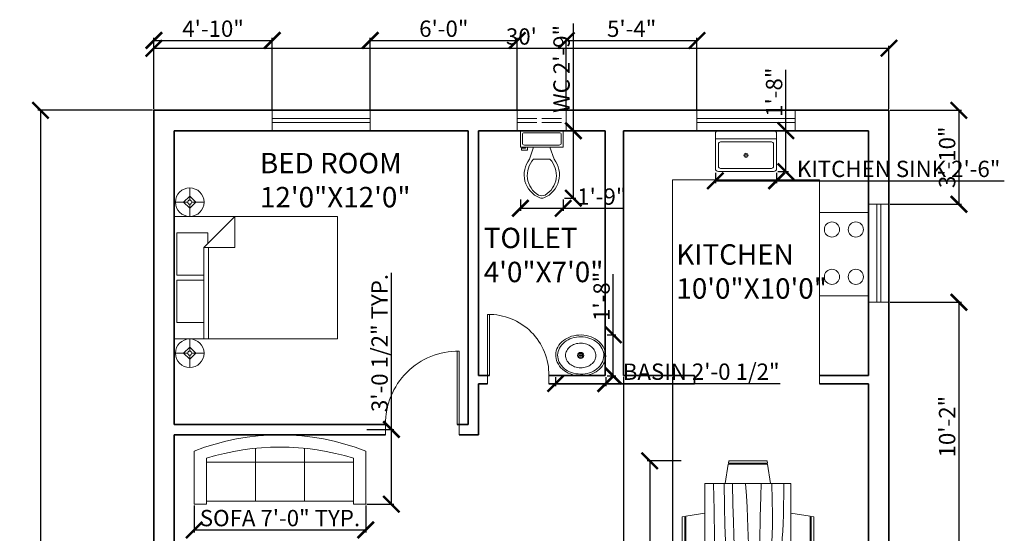
# Model space of a CAD drawing. Units: inches. Extents: x 21865 to 22885, y 36660 to 37408.
# Tile 4 of 6: x 21865 to 22347, y 37157 to 37408. Entities that reach past the tile are written whole.
import ezdxf

# ---------------------------------------------------------------- set-up
doc = ezdxf.new("R2010")
doc.units = ezdxf.units.IN
doc.linetypes.add('ACAD_ISO02W100', pattern=[15, 12, -3])
for name, color, linetype, lineweight in [('A-ANNO-DIMS', 2, 'Continuous', 18), ('A-AREA-IDEN', 7, 'Continuous', 20), ('A-DOOR', 3, 'Continuous', 20), ('A-EQPM', 9, 'Continuous', 18), ('A-FLOR-CASE', 8, 'Continuous', 20), ('A-FLOR-FIXT', 9, 'Continuous', 18), ('A-FURN', 8, 'Continuous', 18), ('A-GLAZ', 4, 'Continuous', 18), ('A-GLAZ-OVHD', 4, 'ACAD_ISO02W100', 18), ('A-WALL', 7, 'Continuous', 35)]:
    doc.layers.add(name, color=color, linetype=linetype, lineweight=lineweight)
doc.styles.get("Standard").update_dxf_attribs({"font": 'arial.ttf'})
doc.dimstyles.new('ISO-25', dxfattribs={"dimtxt": 8, "dimasz": 8, "dimexe": 1.25, "dimexo": 0.625, "dimtad": 1, "dimlunit": 3, "dimtxsty": 'Standard', "dimblk": 'ARCHTICK', "dimcen": 2.5, "dimclrd": 4, "dimclre": 5, "dimclrt": 1, "dimadec": 0, "dimazin": 0, "dimtfac": 1, "dimtmove": 0, "dimatfit": 3, "dimfxl": 1, "dimarcsym": 0})

# ---------------------------------------------------------------- blocks, each defined once
blk = doc.blocks.new('Sink - Oval top')
for p, q in [((-1, 0), (1, 0)), ((0, 1), (0, -1))]:
    blk.add_line(p, q)
for points in [[(-12.23, 0.39, 0.117634), (-11.46, -3.36, 0.104469), (-8.88, -6.8, 0.090016), (-5.08, -9.07, 0.08192), (-0.32, -10.02, 0.08192), (4.49, -9.38, 0.090016), (8.42, -7.36, 0.104469), (11.22, -4.09, 0.117634), (12.23, -0.39, 0.117634), (11.46, 3.36, 0.104469), (8.88, 6.8, 0.090016), (5.08, 9.07, 0.08192), (0.32, 10.02, 0.08192), (-4.49, 9.38, 0.090016), (-8.42, 7.36, 0.104469), (-11.22, 4.09, 0.117634)], [(-11.29, 0.16, 0.118622), (-10.52, -3.25, 0.104678), (-8.07, -6.36, 0.089562), (-4.54, -8.37, 0.081185), (-0.13, -9.15, 0.081185), (4.3, -8.49, 0.089562), (7.89, -6.58, 0.104678), (10.42, -3.55, 0.118622), (11.29, -0.16, 0.118622), (10.52, 3.25, 0.104678), (8.07, 6.36, 0.089562), (4.54, 8.37, 0.081185), (0.13, 9.15, 0.081185), (-4.3, 8.49, 0.089562), (-7.89, 6.58, 0.104678), (-10.42, 3.55, 0.118622)], [(-7.42, 0.08, 0.118283), (-6.91, -2.17, 0.104607), (-5.29, -4.21, 0.089718), (-2.97, -5.53, 0.081436), (-0.07, -6.04, 0.081436), (2.84, -5.59, 0.089718), (5.2, -4.33, 0.104607), (6.86, -2.32, 0.118283), (7.42, -0.08, 0.118283), (6.91, 2.17, 0.104607), (5.29, 4.21, 0.089718), (2.97, 5.53, 0.081436), (0.07, 6.04, 0.081436), (-2.84, 5.59, 0.089718), (-5.2, 4.33, 0.104607), (-6.86, 2.32, 0.118283)]]:
    blk.add_lwpolyline(points, format="xyb", close=True)
for radius in [1.5, 1]:
    blk.add_circle((0, 0), radius)
blk = doc.blocks.new('Toilet - top')
for p, q in [((9.5, -6), (9.5, -2)), ((-10, -8.5), (-8, -8.5)), ((-10, -9.5), (-10, -8.5)), ((-7, -9.5), (-10, -9.5)), ((-8, -8.5), (-8, -8)), ((-7, -8), (-7, -9.5)), ((-4, -8), (-6, -14)), ((4, -8), (6, -14)), ((4, -14), (-4, -14))]:
    blk.add_line(p, q)
blk.add_lwpolyline([(10.5, -8), (10.5, 0), (-10.5, 0), (-10.5, -8)], close=True)
for points in [[(-9.5, -2), (-9.5, -6)], [(8.5, -1), (-8.5, -1)], [(-8.5, -7), (8.5, -7)]]:
    blk.add_lwpolyline(points)
for centre, radius, start, end in [((-8.62, -1.88), 0.884, 81.8699, 188.1301), ((8.62, -1.88), 0.884, 351.8699, 98.1301), ((-8.62, -6.12), 0.884, 171.8699, 278.1301), ((8.62, -6.12), 0.884, 261.8699, 8.1301), ((3.52, -21.58), 12.17, 141.4691, 247.9714), ((4.2, -21.82), 11.33, 136.3677, 238.9468), ((-3.52, -21.58), 12.17, 292.0284, 38.5307), ((-4.2, -21.82), 11.33, 301.053, 43.6321), ((0, -27.88), 4, 245.7318, 294.2682), ((0, -29), 4, 254.8605, 285.1395)]:
    blk.add_arc(centre, radius, start, end)
blk = doc.blocks.new('Sink-single - 30 in top')
blk.add_line((-15, -3.999996), (15, -3.999996))
for points in [[(-13.5, 0), (13.5, 0)], [(-15, -18.499996), (-15, -1.5)], [(15, -1.5), (15, -18.499996)], [(-13.5, -17.499996), (-13.5, -6.499996)], [(-12.5, -5.499996), (12.5, -5.499996)], [(13.5, -6.499996), (13.5, -17.499996)], [(12.5, -18.499996), (-12.5, -18.499996)], [(13.5, -19.999996), (-13.5, -19.999996)]]:
    blk.add_lwpolyline(points)
for radius in [1, 0.5]:
    blk.add_circle((0, -11.999996), radius)
for centre, radius, start, end in [((-13.5, -1.5), 1.5, 90, 180), ((13.5, -1.5), 1.5, 0, 90), ((-12.5, -6.499996), 1, 90, 180), ((12.5, -6.499996), 1, 0, 90), ((-13.5, -18.499996), 1.5, 180, 270), ((-12.5, -17.499996), 1, 180, 270), ((12.5, -17.499996), 1, 270, 0), ((13.5, -18.499996), 1.5, 270, 0)]:
    blk.add_arc(centre, radius, start, end)
blk = doc.blocks.new('Sofa - Roundback 7 ft.')
for p, q in [((-12.00002, -32.4421), (-12.00003, -6.5971)), ((11.99997, -32.4421), (11.99998, -6.5971)), ((-36.000027, -34), (-36.000027, -11.4696)), ((-35.999844, -13.3819), (35.9998, -13.3819)), ((35.99998, -34), (35.99998, -11.4696)), ((-36.000027, -32.4421), (35.99998, -32.4421))]:
    blk.add_line(p, q)
for points in [[(-36.000027, -34), (-42.000027, -34), (-42.000027, -8)], [(41.99998, -8), (41.99998, -34), (35.99998, -34)]]:
    blk.add_lwpolyline(points)
for centre, radius, start, end in [((0, -114.25), 114.25, 68.43141, 111.5686), ((-0.00001, -127.1968), 121.1968, 72.72033, 107.2797)]:
    blk.add_arc(centre, radius, start, end)
blk = doc.blocks.new('Dining Set - 36 x 72 in.')
for p, q in [((-22.2343, 26.00059), (-23.4847, 17.99762)), ((-22.2304, 26), (-5.7608, 26)), ((-22, 27.5), (-22.1562, 26.50042)), ((-5.8416, 26.5), (-22.1534, 26.5)), ((-22, 27.5), (-6, 27.5)), ((-5.8437, 26.49966), (-6, 27.5)), ((-4.5152, 17.99762), (-5.7655, 25.99926)), ((5.7657, 26.00059), (4.5153, 17.99762)), ((5.7696, 26), (22.2392, 26)), ((6, 27.5), (5.8438, 26.50042)), ((22.1584, 26.5), (5.8466, 26.5)), ((6, 27.5), (22, 27.5)), ((22.1563, 26.49966), (22, 27.5)), ((23.4848, 17.99762), (22.2345, 25.99926)), ((36, 18), (-36, 18)), ((-36, 18), (-36, -18)), ((36, -18), (36, 18)), ((-44.0006, 8.23428), (-35.9976, 9.48474)), ((44.0006, 8.23428), (35.9976, 9.48474)), ((-45.5, 8), (-44.5004, 8.15617)), ((-45.5, 8), (-45.5, -8)), ((-44.5, -8.15843), (-44.5, 8.15338)), ((-44, 8.23041), (-44, -8.23915)), ((44, 8.23041), (44, -8.23915)), ((44.5, -8.15843), (44.5, 8.15338)), ((45.5, 8), (44.5005, 8.15617)), ((45.5, 8), (45.5, -8)), ((-44.4997, -8.15631), (-45.5, -8)), ((-35.9976, -9.48476), (-43.9993, -8.2345)), ((35.9976, -9.48476), (43.9993, -8.2345)), ((44.4997, -8.15631), (45.5, -8)), ((-36, -18), (36, -18)), ((-22.2343, -26.0006), (-23.4847, -17.99762)), ((-4.5152, -17.99762), (-5.7655, -25.99928)), ((5.7657, -26.0006), (4.5153, -17.99762)), ((23.4848, -17.99762), (22.2345, -25.99928)), ((-22.2304, -26), (-5.7608, -26)), ((-22, -27.5), (-22.1562, -26.50044)), ((-5.8416, -26.5), (-22.1534, -26.5)), ((-22, -27.5), (-6, -27.5)), ((-5.8437, -26.49967), (-6, -27.5)), ((5.7696, -26), (22.2392, -26)), ((6, -27.5), (5.8438, -26.50044)), ((22.1584, -26.5), (5.8466, -26.5)), ((6, -27.5), (22, -27.5)), ((22.1563, -26.49967), (22, -27.5))]:
    blk.add_line(p, q)
for points in [[(-36, 15), (-31.1772, 14.97754), (-26.8079, 14.91406), (-22.8538, 14.81543), (-19.276, 14.6875), (-16.0362, 14.53613), (-13.0957, 14.36718), (-10.4159, 14.18652), (-7.9583, 14), (-5.6904, 13.81315), (-3.6035, 13.63021), (-1.6954, 13.45508), (0.0365, 13.29166), (1.5945, 13.14388), (2.9811, 13.01562), (4.1988, 12.9108), (5.25, 12.83333), (6.1393, 12.78613), (6.8802, 12.76823), (7.4883, 12.77767), (7.9792, 12.8125), (8.3685, 12.87077), (8.6719, 12.95052), (8.9049, 13.0498), (9.0833, 13.16666), (9.2205, 13.29899), (9.3216, 13.44401), (9.3895, 13.59879), (9.4271, 13.76041), (9.4373, 13.92594), (9.4232, 14.09245), (9.3875, 14.257), (9.3333, 14.41666), (9.2638, 14.56917), (9.1836, 14.71484), (9.0975, 14.85465), (9.0104, 14.98958), (8.9272, 15.1206), (8.8529, 15.2487), (8.7922, 15.37483), (8.75, 15.5), (8.7305, 15.62467), (8.7344, 15.74739), (8.7617, 15.86621), (8.8125, 15.97916), (8.8867, 16.08431), (8.9844, 16.17968), (9.1055, 16.26334), (9.25, 16.33333), (9.4189, 16.38802), (9.6172, 16.42708), (9.8506, 16.45052), (10.125, 16.45833), (10.4463, 16.45052), (10.8203, 16.42708), (11.2529, 16.38802), (11.75, 16.33333), (12.3184, 16.26318), (12.9694, 16.17838), (13.7151, 16.07991), (14.5677, 15.96875), (15.5395, 15.84586), (16.6426, 15.71224), (17.8893, 15.56884), (19.2917, 15.41666), (20.859, 15.25667), (22.5879, 15.08984), (24.4721, 14.91715), (26.5052, 14.73958), (28.6809, 14.5581), (30.9929, 14.3737), (33.4347, 14.18733), (36, 14)], [(-36, 10), (-28.9766, 10.14274), (-23.1725, 10.20442), (-18.4241, 10.19775), (-14.5677, 10.13541), (-11.4399, 10.03011), (-8.877, 9.89453), (-6.7154, 9.74137), (-4.7917, 9.58333), (-2.9698, 9.43082), (-1.2246, 9.28515), (0.4415, 9.14534), (2.026, 9.01041), (3.5266, 8.87939), (4.9408, 8.7513), (6.266, 8.62516), (7.5, 8.5), (8.6411, 8.37549), (9.6914, 8.2539), (10.6538, 8.13818), (11.5312, 8.03125), (12.3267, 7.93603), (13.043, 7.85547), (13.6831, 7.79248), (14.25, 7.75), (14.7471, 7.7303), (15.1797, 7.73307), (15.5537, 7.75732), (15.875, 7.80208), (16.1494, 7.86637), (16.3828, 7.94922), (16.5811, 8.04964), (16.75, 8.16666), (16.8944, 8.29915), (17.0143, 8.44531), (17.1089, 8.60319), (17.1771, 8.77083), (17.218, 8.94629), (17.2305, 9.1276), (17.2137, 9.31282), (17.1667, 9.5), (17.0895, 9.6875), (16.987, 9.875), (16.8649, 10.0625), (16.7292, 10.25), (16.5856, 10.4375), (16.4401, 10.625), (16.2985, 10.8125), (16.1667, 11), (16.05, 11.18733), (15.9518, 11.3737), (15.8752, 11.5581), (15.8229, 11.73958), (15.798, 11.91715), (15.8034, 12.08984), (15.842, 12.25667), (15.9167, 12.41666), (16.0295, 12.56836), (16.1784, 12.70833), (16.3605, 12.83268), (16.5729, 12.9375), (16.8127, 13.01888), (17.0768, 13.07291), (17.3625, 13.0957), (17.6667, 13.08333), (17.9894, 13.03312), (18.3418, 12.94726), (18.7382, 12.82918), (19.1927, 12.68229), (19.7195, 12.51001), (20.3327, 12.31575), (21.0465, 12.10294), (21.875, 11.875), (22.8357, 11.63354), (23.959, 11.37304), (25.2786, 11.08618), (26.8282, 10.76562), (28.6414, 10.40405), (30.752, 9.99414), (33.1936, 9.52856), (36, 9)], [(-36, 5.5), (-30.7157, 5.3348), (-26.069, 5.20963), (-21.9946, 5.11767), (-18.4271, 5.05208), (-15.3009, 5.00602), (-12.5508, 4.97265), (-10.1112, 4.94515), (-7.9167, 4.91666), (-5.909, 4.88167), (-4.0586, 4.83984), (-2.3429, 4.79215), (-0.7396, 4.73958), (0.7739, 4.6831), (2.22, 4.6237), (3.6213, 4.56233), (5, 4.5), (6.373, 4.43782), (7.7344, 4.3776), (9.0723, 4.32129), (10.375, 4.27083), (11.6309, 4.22819), (12.8281, 4.19531), (13.9551, 4.17415), (15, 4.16666), (15.954, 4.17448), (16.819, 4.19791), (17.6001, 4.23698), (18.3021, 4.29166), (18.9299, 4.36198), (19.4883, 4.44791), (19.9823, 4.54948), (20.4167, 4.66666), (20.7969, 4.79899), (21.1302, 4.94401), (21.4245, 5.09879), (21.6875, 5.26041), (21.9271, 5.42594), (22.1511, 5.59245), (22.3672, 5.757), (22.5834, 5.91666), (22.8065, 6.06868), (23.0404, 6.21093), (23.2879, 6.34147), (23.5521, 6.45833), (23.8358, 6.55957), (24.142, 6.64323), (24.4735, 6.70735), (24.8334, 6.75), (25.2235, 6.76969), (25.642, 6.76692), (26.0858, 6.74267), (26.5521, 6.69791), (27.0379, 6.63362), (27.5404, 6.55078), (28.0565, 6.45036), (28.5834, 6.33333), (29.1242, 6.19987), (29.7071, 6.04687), (30.3661, 5.87044), (31.1354, 5.66666), (32.0493, 5.43164), (33.142, 5.16146), (34.4475, 4.85221), (36, 4.5)], [(-36, -1), (-30.7915, -0.6591), (-26.0195, -0.38216), (-21.6519, -0.16284), (-17.6563, 0.00521), (-14.0005, 0.12833), (-10.6523, 0.21289), (-7.5796, 0.26522), (-4.75, 0.29166), (-2.134, 0.29793), (0.2878, 0.28711), (2.5317, 0.26163), (4.6146, 0.22396), (6.5529, 0.17651), (8.3633, 0.12174), (10.0623, 0.06209), (11.6667, 0), (13.1899, -0.06201), (14.6341, -0.1211), (15.9982, -0.17432), (17.2813, -0.21875), (18.4823, -0.25147), (19.6003, -0.26953), (20.6343, -0.27002), (21.5834, -0.25), (22.4481, -0.20768), (23.2357, -0.14584), (23.9549, -0.06836), (24.6146, 0.02083), (25.2235, 0.11784), (25.7904, 0.21875), (26.3241, 0.31966), (26.8334, 0.41666), (27.3265, 0.50618), (27.8099, 0.58593), (28.2894, 0.65397), (28.7709, 0.70833), (29.2601, 0.74707), (29.763, 0.76823), (30.2855, 0.76985), (30.8334, 0.75), (31.4088, 0.70784), (31.9994, 0.64713), (32.589, 0.57275), (33.1615, 0.48958), (33.7008, 0.4025), (34.1908, 0.3164), (34.6153, 0.23616), (34.9584, 0.16666), (35.2099, 0.11165), (35.3848, 0.07031), (35.504, 0.04069), (35.5886, 0.02083), (35.6594, 0.00879), (35.7377, 0.0026), (35.8442, 0.00032), (36, 0)], [(-36, -6.5), (-27.1843, -6.31267), (-20.084, -6.1263), (-14.469, -5.9419), (-10.1094, -5.76042), (-6.7752, -5.58285), (-4.2363, -5.41016), (-2.2629, -5.24333), (-0.625, -5.08334), (0.8708, -4.93099), (2.2715, -4.78646), (3.5872, -4.64974), (4.8281, -4.52084), (6.0046, -4.39974), (7.127, -4.28646), (8.2053, -4.18099), (9.25, -4.08334), (10.2705, -3.99382), (11.2734, -3.91407), (12.2647, -3.84603), (13.25, -3.79167), (14.2354, -3.75293), (15.2266, -3.73177), (16.2295, -3.73015), (17.25, -3.75), (18.2912, -3.79248), (19.3451, -3.85547), (20.4009, -3.93604), (21.4479, -4.03125), (22.4754, -4.13819), (23.4727, -4.25391), (24.4289, -4.37549), (25.3334, -4.5), (26.1785, -4.62492), (26.9694, -4.74935), (27.7145, -4.87281), (28.4219, -4.99479), (29.1, -5.11483), (29.7572, -5.23242), (30.4016, -5.34709), (31.0417, -5.45834), (31.6837, -5.56437), (32.3262, -5.65821), (32.9658, -5.73153), (33.599, -5.77604), (34.2224, -5.78345), (34.8327, -5.74545), (35.4264, -5.65373), (36, -5.5)], [(-36, -10), (-26.4022, -9.81299), (-18.4675, -9.62891), (-11.9839, -9.45069), (-6.7396, -9.28125), (-2.5226, -9.12354), (0.8789, -8.98047), (3.6769, -8.85498), (6.0833, -8.75), (8.2767, -8.66765), (10.3021, -8.60677), (12.1712, -8.56543), (13.8958, -8.54167), (15.4876, -8.53353), (16.9583, -8.53907), (18.3197, -8.55632), (19.5834, -8.58334), (20.7616, -8.61841), (21.8685, -8.66081), (22.9188, -8.71004), (23.9271, -8.76563), (24.9081, -8.82707), (25.8763, -8.89388), (26.8465, -8.96558), (27.8334, -9.04167), (28.8474, -9.12118), (29.8828, -9.20117), (30.93, -9.27824), (31.9792, -9.34896), (33.0205, -9.40991), (34.0443, -9.45768), (35.0407, -9.48885), (36, -9.5)], [(-36, -14.5), (-30.0881, -14.33513), (-25.0332, -14.21224), (-20.7312, -14.12647), (-17.0781, -14.07292), (-13.97, -14.04671), (-11.3027, -14.04297), (-8.9724, -14.05681), (-6.875, -14.08334), (-4.9224, -14.11833), (-3.0905, -14.16016), (-1.3709, -14.20785), (0.2448, -14.26042), (1.7647, -14.3169), (3.1973, -14.3763), (4.5507, -14.43767), (5.8333, -14.5), (7.0554, -14.5621), (8.235, -14.62175), (9.3922, -14.67652), (10.5469, -14.72396), (11.7192, -14.76164), (12.929, -14.78711), (14.1965, -14.79794), (15.5417, -14.79167), (16.9933, -14.76424), (18.6152, -14.70508), (20.4804, -14.60197), (22.6615, -14.44271), (25.2312, -14.21509), (28.2624, -13.9069), (31.8277, -13.50594), (36, -13)]]:
    blk.add_lwpolyline(points)
blk = doc.blocks.new('Bed - Queen')
for p, q in [((0, -80.00003), (0, 0)), ((0, 0), (59.99999, 0)), ((59.99999, 0), (59.99999, -80.00003)), ((7.99999, -1.2), (28.79998, -1.2)), ((7.99999, -14.4), (7.99999, -1.2)), ((28.79998, -1.2), (28.79998, -14.4)), ((31.19999, -1.2), (51.99999, -1.2)), ((31.19999, -14.4), (31.19999, -1.2)), ((51.99999, -1.2), (51.99999, -16.4)), ((0, -14.4), (44.8, -14.4)), ((59.99999, -29.6), (44.8, -14.4)), ((44.8, -14.4), (44.8, -29.6)), ((44.8, -16.8), (0, -16.8)), ((51.99999, -16.4), (46.79936, -16.4)), ((44.8, -29.6), (59.99999, -29.6)), ((59.99999, -80.00003), (0, -80.00003))]:
    blk.add_line(p, q)
blk = doc.blocks.new('Lamp - Table')
for p, q in [((0, 7), (0, 1)), ((-1, 0), (-7, 0)), ((0, 3), (-3, 0)), ((-3, 0), (0, -3)), ((3, 0), (0, 3)), ((0, -3), (3, 0)), ((1, 0), (7, 0)), ((0, -1), (0, -7))]:
    blk.add_line(p, q)
for radius in [7, 1]:
    blk.add_circle((0, 0), radius)
blk = doc.blocks.new('new block')
for name, p in [('Lamp - Table', (-35.8, -6.38)), ('Bed - Queen', (-28.8, 1.2))]:
    blk.add_blockref(name, p)
at = {"xscale": -1}
blk.add_blockref('Lamp - Table', (38.2, -6.38), dxfattribs=at)
blk = doc.blocks.new('_ArchTick')
at = {"color": 0, "linetype": 'ByBlock', "const_width": 0.15}
blk.add_lwpolyline([(-0.5, -0.5), (0.5, 0.5)], dxfattribs=at)
blk = doc.blocks.new('*D21')
at = {"layer": 'A-ANNO-DIMS', "color": 0, "lineweight": -2, "transparency": 16777216}
for p, q in [((21930.43, 37364.56), (21930.43, 37395.61)), ((21930.43, 37394.36), (22290.43, 37394.36)), ((22290.43, 37364.56), (22290.43, 37395.61))]:
    blk.add_line(p, q, dxfattribs=at)
at = {"layer": 'Defpoints', "color": 0, "transparency": 16777216}
for p in [(22290.43, 37394.36), (21930.43, 37363.93), (22290.43, 37363.93)]:
    blk.add_point(p, dxfattribs=at)
at = {"layer": 'A-ANNO-DIMS', "color": 0, "lineweight": -2, "transparency": 16777216, "xscale": 8, "yscale": 8, "zscale": 8, "rotation": 180}
blk.add_blockref('_ArchTick', (21930.43, 37394.36), dxfattribs=at)
at = {"layer": 'A-ANNO-DIMS', "color": 0, "lineweight": -2, "transparency": 16777216, "xscale": 8, "yscale": 8, "zscale": 8}
blk.add_blockref('_ArchTick', (22290.43, 37394.36), dxfattribs=at)
at = {"layer": 'A-ANNO-DIMS', "color": 0, "transparency": 16777216, "insert": (22110.43, 37399.07), "char_height": 8, "attachment_point": 5}
blk.add_mtext("30'", dxfattribs=at)
blk = doc.blocks.new('*D22')
at = {"layer": 'A-ANNO-DIMS', "color": 0, "lineweight": -2, "transparency": 16777216}
for p, q in [((21929.8, 37363.93), (21873.63, 37363.93)), ((21874.88, 37363.93), (21874.88, 36883.93)), ((21929.8, 36883.93), (21873.63, 36883.93))]:
    blk.add_line(p, q, dxfattribs=at)
at = {"layer": 'Defpoints', "color": 0, "transparency": 16777216}
for p in [(21930.43, 37363.93), (21874.88, 36883.93), (21930.43, 36883.93)]:
    blk.add_point(p, dxfattribs=at)
at = {"layer": 'A-ANNO-DIMS', "color": 0, "lineweight": -2, "transparency": 16777216, "xscale": 8, "yscale": 8, "zscale": 8}
for p, rotation in [((21874.88, 37363.93), 90), ((21874.88, 36883.93), 270)]:
    blk.add_blockref('_ArchTick', p, dxfattribs=dict(at, rotation=rotation))
at = {"layer": 'A-ANNO-DIMS', "color": 0, "transparency": 16777216, "insert": (21870.17, 37123.93), "char_height": 8, "attachment_point": 5, "rotation": 90}
blk.add_mtext("40'", dxfattribs=at)
blk = doc.blocks.new('WIN-W-48-PLAN')
for p, q in [((0, 0), (0, 10)), ((48, 0), (48, 10)), ((48, 6), (0, 6)), ((48, 4), (0, 4))]:
    blk.add_line(p, q)
blk = doc.blocks.new('DOOR-D1-36-PLAN')
for p, q in [((0, 36), (0, 41)), ((36, 36), (36, 41)), ((35, 36), (35, 0)), ((36, 36), (36, 0))]:
    blk.add_line(p, q)
blk.add_arc((35.5, 35.5), 35.5, 179.1931, 270.8069)
blk = doc.blocks.new('*D32')
at = {"layer": 'A-ANNO-DIMS', "color": 5, "lineweight": -2, "transparency": 16777216}
for p, q in [((21950.18, 37170.31), (21950.18, 37157.08)), ((22034.18, 37170.31), (22034.18, 37157.08))]:
    blk.add_line(p, q, dxfattribs=at)
at = {"layer": 'A-ANNO-DIMS', "color": 4, "lineweight": -2, "transparency": 16777216}
blk.add_line((21950.18, 37158.33), (22034.18, 37158.33), dxfattribs=at)
at = {"layer": 'Defpoints', "color": 0, "transparency": 16777216}
for p in [(21950.18, 37170.93), (22034.18, 37170.93), (22034.18, 37158.33)]:
    blk.add_point(p, dxfattribs=at)
at = {"layer": 'A-ANNO-DIMS', "color": 4, "lineweight": -2, "transparency": 16777216, "xscale": 8, "yscale": 8, "zscale": 8, "rotation": 180}
blk.add_blockref('_ArchTick', (21950.18, 37158.33), dxfattribs=at)
at = {"layer": 'A-ANNO-DIMS', "color": 4, "lineweight": -2, "transparency": 16777216, "xscale": 8, "yscale": 8, "zscale": 8}
blk.add_blockref('_ArchTick', (22034.18, 37158.33), dxfattribs=at)
at = {"layer": 'A-ANNO-DIMS', "color": 1, "transparency": 16777216, "insert": (21992.18, 37163.1), "char_height": 8, "attachment_point": 5}
blk.add_mtext('SOFA 7\'-0" TYP.', dxfattribs=at)
blk = doc.blocks.new('*D33')
at = {"layer": 'A-ANNO-DIMS', "color": 4, "lineweight": -2, "transparency": 16777216}
for p, q in [((22046.78, 37207.6), (22046.78, 37284.25)), ((22046.78, 37170.93), (22046.78, 37207.6))]:
    blk.add_line(p, q, dxfattribs=at)
at = {"layer": 'A-ANNO-DIMS', "color": 5, "lineweight": -2, "transparency": 16777216}
for p, q in [((22034.8, 37207.6), (22048.03, 37207.6)), ((22034.8, 37170.93), (22048.03, 37170.93))]:
    blk.add_line(p, q, dxfattribs=at)
at = {"layer": 'Defpoints', "color": 0, "transparency": 16777216}
for p in [(22034.18, 37207.6), (22046.78, 37207.6), (22034.18, 37170.93)]:
    blk.add_point(p, dxfattribs=at)
at = {"layer": 'A-ANNO-DIMS', "color": 4, "lineweight": -2, "transparency": 16777216, "xscale": 8, "yscale": 8, "zscale": 8}
for p, rotation in [((22046.78, 37207.6), 90), ((22046.78, 37170.93), 270)]:
    blk.add_blockref('_ArchTick', p, dxfattribs=dict(at, rotation=rotation))
at = {"layer": 'A-ANNO-DIMS', "color": 1, "transparency": 16777216, "insert": (22042.02, 37249.92), "char_height": 8, "attachment_point": 5, "rotation": 90}
blk.add_mtext('3\'-0 1/2" TYP.', dxfattribs=at)
blk = doc.blocks.new('*D42')
at = {"layer": 'A-ANNO-DIMS', "color": 5, "lineweight": -2, "transparency": 16777216}
for p, q in [((22127.21, 37233.13), (22127.21, 37228.83)), ((22151.76, 37233.13), (22151.76, 37228.83))]:
    blk.add_line(p, q, dxfattribs=at)
at = {"layer": 'A-ANNO-DIMS', "color": 4, "lineweight": -2, "transparency": 16777216}
for p, q in [((22127.21, 37230.08), (22151.76, 37230.08)), ((22151.76, 37230.08), (22237.21, 37230.08))]:
    blk.add_line(p, q, dxfattribs=at)
at = {"layer": 'Defpoints', "color": 0, "transparency": 16777216}
for p in [(22127.21, 37233.76), (22151.76, 37233.76), (22151.76, 37230.08)]:
    blk.add_point(p, dxfattribs=at)
at = {"layer": 'A-ANNO-DIMS', "color": 4, "lineweight": -2, "transparency": 16777216, "xscale": 8, "yscale": 8, "zscale": 8, "rotation": 180}
blk.add_blockref('_ArchTick', (22127.21, 37230.08), dxfattribs=at)
at = {"layer": 'A-ANNO-DIMS', "color": 4, "lineweight": -2, "transparency": 16777216, "xscale": 8, "yscale": 8, "zscale": 8}
blk.add_blockref('_ArchTick', (22151.76, 37230.08), dxfattribs=at)
at = {"layer": 'A-ANNO-DIMS', "color": 1, "transparency": 16777216, "insert": (22198.48, 37234.84), "char_height": 8, "attachment_point": 5}
blk.add_mtext('BASIN 2\'-0 1/2"', dxfattribs=at)
blk = doc.blocks.new('*D43')
at = {"layer": 'A-ANNO-DIMS', "color": 4, "lineweight": -2, "transparency": 16777216}
for p, q in [((22155.44, 37253.9), (22155.44, 37283.66)), ((22155.44, 37233.76), (22155.44, 37253.9))]:
    blk.add_line(p, q, dxfattribs=at)
at = {"layer": 'A-ANNO-DIMS', "color": 5, "lineweight": -2, "transparency": 16777216}
for p, q in [((22152.38, 37253.9), (22156.69, 37253.9)), ((22152.38, 37233.76), (22156.69, 37233.76))]:
    blk.add_line(p, q, dxfattribs=at)
at = {"layer": 'Defpoints', "color": 0, "transparency": 16777216}
for p in [(22151.76, 37253.9), (22155.44, 37253.9), (22151.76, 37233.76)]:
    blk.add_point(p, dxfattribs=at)
at = {"layer": 'A-ANNO-DIMS', "color": 4, "lineweight": -2, "transparency": 16777216, "xscale": 8, "yscale": 8, "zscale": 8}
for p, rotation in [((22155.44, 37253.9), 90), ((22155.44, 37233.76), 270)]:
    blk.add_blockref('_ArchTick', p, dxfattribs=dict(at, rotation=rotation))
at = {"layer": 'A-ANNO-DIMS', "color": 1, "transparency": 16777216, "insert": (22150.73, 37272.78), "char_height": 8, "attachment_point": 5, "rotation": 90}
blk.add_mtext('1\'-8"', dxfattribs=at)
blk = doc.blocks.new('*D44')
at = {"layer": 'A-ANNO-DIMS', "color": 4, "lineweight": -2, "transparency": 16777216}
for p, q in [((22135.89, 37353.93), (22135.89, 37406.5)), ((22135.89, 37320.89), (22135.89, 37353.93))]:
    blk.add_line(p, q, dxfattribs=at)
at = {"layer": 'A-ANNO-DIMS', "color": 5, "lineweight": -2, "transparency": 16777216}
for p, q in [((22131.55, 37353.93), (22137.14, 37353.93)), ((22131.55, 37320.89), (22137.14, 37320.89))]:
    blk.add_line(p, q, dxfattribs=at)
at = {"layer": 'Defpoints', "color": 0, "transparency": 16777216}
for p in [(22130.93, 37353.93), (22135.89, 37353.93), (22130.93, 37320.89)]:
    blk.add_point(p, dxfattribs=at)
at = {"layer": 'A-ANNO-DIMS', "color": 4, "lineweight": -2, "transparency": 16777216, "xscale": 8, "yscale": 8, "zscale": 8}
for p, rotation in [((22135.89, 37353.93), 90), ((22135.89, 37320.89), 270)]:
    blk.add_blockref('_ArchTick', p, dxfattribs=dict(at, rotation=rotation))
at = {"layer": 'A-ANNO-DIMS', "color": 1, "transparency": 16777216, "insert": (22131.13, 37384.22), "char_height": 8, "attachment_point": 5, "rotation": 90}
blk.add_mtext('WC 2\'-9"', dxfattribs=at)
blk = doc.blocks.new('*D45')
at = {"layer": 'A-ANNO-DIMS', "color": 5, "lineweight": -2, "transparency": 16777216}
for p, q in [((22109.93, 37320.26), (22109.93, 37314.68)), ((22130.93, 37320.26), (22130.93, 37314.68))]:
    blk.add_line(p, q, dxfattribs=at)
at = {"layer": 'A-ANNO-DIMS', "color": 4, "lineweight": -2, "transparency": 16777216}
for p, q in [((22109.93, 37315.93), (22130.93, 37315.93)), ((22130.93, 37315.93), (22160.69, 37315.93))]:
    blk.add_line(p, q, dxfattribs=at)
at = {"layer": 'Defpoints', "color": 0, "transparency": 16777216}
for p in [(22109.93, 37320.89), (22130.93, 37320.89), (22130.93, 37315.93)]:
    blk.add_point(p, dxfattribs=at)
at = {"layer": 'A-ANNO-DIMS', "color": 4, "lineweight": -2, "transparency": 16777216, "xscale": 8, "yscale": 8, "zscale": 8, "rotation": 180}
blk.add_blockref('_ArchTick', (22109.93, 37315.93), dxfattribs=at)
at = {"layer": 'A-ANNO-DIMS', "color": 4, "lineweight": -2, "transparency": 16777216, "xscale": 8, "yscale": 8, "zscale": 8}
blk.add_blockref('_ArchTick', (22130.93, 37315.93), dxfattribs=at)
at = {"layer": 'A-ANNO-DIMS', "color": 1, "transparency": 16777216, "insert": (22149.81, 37320.64), "char_height": 8, "attachment_point": 5}
blk.add_mtext('1\'-9"', dxfattribs=at)
blk = doc.blocks.new('*D46')
at = {"layer": 'A-ANNO-DIMS', "color": 5, "lineweight": -2, "transparency": 16777216}
for p, q in [((22205.43, 37333.31), (22205.43, 37328.18)), ((22235.43, 37333.31), (22235.43, 37328.18))]:
    blk.add_line(p, q, dxfattribs=at)
at = {"layer": 'A-ANNO-DIMS', "color": 4, "lineweight": -2, "transparency": 16777216}
for p, q in [((22205.43, 37329.43), (22235.43, 37329.43)), ((22235.43, 37329.43), (22346.94, 37329.43))]:
    blk.add_line(p, q, dxfattribs=at)
at = {"layer": 'Defpoints', "color": 0, "transparency": 16777216}
for p in [(22205.43, 37333.93), (22235.43, 37333.93), (22235.43, 37329.43)]:
    blk.add_point(p, dxfattribs=at)
at = {"layer": 'A-ANNO-DIMS', "color": 4, "lineweight": -2, "transparency": 16777216, "xscale": 8, "yscale": 8, "zscale": 8, "rotation": 180}
blk.add_blockref('_ArchTick', (22205.43, 37329.43), dxfattribs=at)
at = {"layer": 'A-ANNO-DIMS', "color": 4, "lineweight": -2, "transparency": 16777216, "xscale": 8, "yscale": 8, "zscale": 8}
blk.add_blockref('_ArchTick', (22235.43, 37329.43), dxfattribs=at)
at = {"layer": 'A-ANNO-DIMS', "color": 1, "transparency": 16777216, "insert": (22295.18, 37334.19), "char_height": 8, "attachment_point": 5}
blk.add_mtext('KITCHEN SINK 2\'-6"', dxfattribs=at)
blk = doc.blocks.new('*D47')
at = {"layer": 'A-ANNO-DIMS', "color": 4, "lineweight": -2, "transparency": 16777216}
for p, q in [((22239.93, 37353.93), (22239.93, 37383.69)), ((22239.93, 37333.93), (22239.93, 37353.93))]:
    blk.add_line(p, q, dxfattribs=at)
at = {"layer": 'A-ANNO-DIMS', "color": 5, "lineweight": -2, "transparency": 16777216}
for p, q in [((22236.05, 37353.93), (22241.18, 37353.93)), ((22236.05, 37333.93), (22241.18, 37333.93))]:
    blk.add_line(p, q, dxfattribs=at)
at = {"layer": 'Defpoints', "color": 0, "transparency": 16777216}
for p in [(22235.43, 37353.93), (22239.93, 37353.93), (22235.43, 37333.93)]:
    blk.add_point(p, dxfattribs=at)
at = {"layer": 'A-ANNO-DIMS', "color": 4, "lineweight": -2, "transparency": 16777216, "xscale": 8, "yscale": 8, "zscale": 8}
for p, rotation in [((22239.93, 37353.93), 90), ((22239.93, 37333.93), 270)]:
    blk.add_blockref('_ArchTick', p, dxfattribs=dict(at, rotation=rotation))
at = {"layer": 'A-ANNO-DIMS', "color": 1, "transparency": 16777216, "insert": (22235.22, 37372.81), "char_height": 8, "attachment_point": 5, "rotation": 90}
blk.add_mtext('1\'-8"', dxfattribs=at)
blk = doc.blocks.new('*D48')
at = {"layer": 'A-ANNO-DIMS', "color": 5, "lineweight": -2, "transparency": 16777216}
for p, q in [((22188.6, 37192.23), (22172.01, 37192.23)), ((22188.6, 37085.76), (22172.01, 37085.76))]:
    blk.add_line(p, q, dxfattribs=at)
at = {"layer": 'A-ANNO-DIMS', "color": 4, "lineweight": -2, "transparency": 16777216}
for p, q in [((22173.26, 37192.23), (22173.26, 37085.76)), ((22173.26, 37085.76), (22173.26, 36963.72))]:
    blk.add_line(p, q, dxfattribs=at)
at = {"layer": 'Defpoints', "color": 0, "transparency": 16777216}
for p in [(22189.23, 37192.23), (22173.26, 37085.76), (22189.23, 37085.76)]:
    blk.add_point(p, dxfattribs=at)
at = {"layer": 'A-ANNO-DIMS', "color": 4, "lineweight": -2, "transparency": 16777216, "xscale": 8, "yscale": 8, "zscale": 8}
for p, rotation in [((22173.26, 37192.23), 90), ((22173.26, 37085.76), 270)]:
    blk.add_blockref('_ArchTick', p, dxfattribs=dict(at, rotation=rotation))
at = {"layer": 'A-ANNO-DIMS', "color": 1, "transparency": 16777216, "insert": (22168.49, 37020.74), "char_height": 8, "attachment_point": 5, "rotation": 90}
blk.add_mtext('DINING SET 8\'-10 1/2"', dxfattribs=at)
blk = doc.blocks.new('*D52')
at = {"layer": 'A-ANNO-DIMS', "color": 5, "lineweight": -2, "transparency": 16777216}
for p, q in [((21930.43, 37364.56), (21930.43, 37399.43)), ((21988.43, 37364.56), (21988.43, 37399.43))]:
    blk.add_line(p, q, dxfattribs=at)
at = {"layer": 'A-ANNO-DIMS', "color": 4, "lineweight": -2, "transparency": 16777216}
blk.add_line((21930.43, 37398.18), (21988.43, 37398.18), dxfattribs=at)
at = {"layer": 'Defpoints', "color": 0, "transparency": 16777216}
for p in [(21988.43, 37398.18), (21930.43, 37363.93), (21988.43, 37363.93)]:
    blk.add_point(p, dxfattribs=at)
at = {"layer": 'A-ANNO-DIMS', "color": 4, "lineweight": -2, "transparency": 16777216, "xscale": 8, "yscale": 8, "zscale": 8, "rotation": 180}
blk.add_blockref('_ArchTick', (21930.43, 37398.18), dxfattribs=at)
at = {"layer": 'A-ANNO-DIMS', "color": 4, "lineweight": -2, "transparency": 16777216, "xscale": 8, "yscale": 8, "zscale": 8}
blk.add_blockref('_ArchTick', (21988.43, 37398.18), dxfattribs=at)
at = {"layer": 'A-ANNO-DIMS', "color": 1, "transparency": 16777216, "insert": (21959.43, 37402.89), "char_height": 8, "attachment_point": 5}
blk.add_mtext('4\'-10"', dxfattribs=at)
blk = doc.blocks.new('*D53')
at = {"layer": 'A-ANNO-DIMS', "color": 5, "lineweight": -2, "transparency": 16777216}
for p, q in [((22036.43, 37364.56), (22036.43, 37399.43)), ((22108.43, 37364.56), (22108.43, 37399.43))]:
    blk.add_line(p, q, dxfattribs=at)
at = {"layer": 'A-ANNO-DIMS', "color": 4, "lineweight": -2, "transparency": 16777216}
blk.add_line((22036.43, 37398.18), (22108.43, 37398.18), dxfattribs=at)
at = {"layer": 'Defpoints', "color": 0, "transparency": 16777216}
for p in [(22108.43, 37398.18), (22036.43, 37363.93), (22108.43, 37363.93)]:
    blk.add_point(p, dxfattribs=at)
at = {"layer": 'A-ANNO-DIMS', "color": 4, "lineweight": -2, "transparency": 16777216, "xscale": 8, "yscale": 8, "zscale": 8, "rotation": 180}
blk.add_blockref('_ArchTick', (22036.43, 37398.18), dxfattribs=at)
at = {"layer": 'A-ANNO-DIMS', "color": 4, "lineweight": -2, "transparency": 16777216, "xscale": 8, "yscale": 8, "zscale": 8}
blk.add_blockref('_ArchTick', (22108.43, 37398.18), dxfattribs=at)
at = {"layer": 'A-ANNO-DIMS', "color": 1, "transparency": 16777216, "insert": (22072.43, 37402.89), "char_height": 8, "attachment_point": 5}
blk.add_mtext('6\'-0"', dxfattribs=at)
blk = doc.blocks.new('*D54')
at = {"layer": 'A-ANNO-DIMS', "color": 5, "lineweight": -2, "transparency": 16777216}
for p, q in [((22132.43, 37364.56), (22132.43, 37399.43)), ((22196.43, 37364.56), (22196.43, 37399.43))]:
    blk.add_line(p, q, dxfattribs=at)
at = {"layer": 'A-ANNO-DIMS', "color": 4, "lineweight": -2, "transparency": 16777216}
blk.add_line((22132.43, 37398.18), (22196.43, 37398.18), dxfattribs=at)
at = {"layer": 'Defpoints', "color": 0, "transparency": 16777216}
for p in [(22196.43, 37398.18), (22132.43, 37363.93), (22196.43, 37363.93)]:
    blk.add_point(p, dxfattribs=at)
at = {"layer": 'A-ANNO-DIMS', "color": 4, "lineweight": -2, "transparency": 16777216, "xscale": 8, "yscale": 8, "zscale": 8, "rotation": 180}
blk.add_blockref('_ArchTick', (22132.43, 37398.18), dxfattribs=at)
at = {"layer": 'A-ANNO-DIMS', "color": 4, "lineweight": -2, "transparency": 16777216, "xscale": 8, "yscale": 8, "zscale": 8}
blk.add_blockref('_ArchTick', (22196.43, 37398.18), dxfattribs=at)
at = {"layer": 'A-ANNO-DIMS', "color": 1, "transparency": 16777216, "insert": (22164.43, 37402.87), "char_height": 8, "attachment_point": 5}
blk.add_mtext('5\'-4"', dxfattribs=at)
blk = doc.blocks.new('*D56')
at = {"layer": 'A-ANNO-DIMS', "color": 5, "lineweight": -2, "transparency": 16777216}
for p, q in [((22291.05, 37363.93), (22325.93, 37363.93)), ((22291.05, 37317.93), (22325.93, 37317.93))]:
    blk.add_line(p, q, dxfattribs=at)
at = {"layer": 'A-ANNO-DIMS', "color": 4, "lineweight": -2, "transparency": 16777216}
blk.add_line((22324.68, 37363.93), (22324.68, 37317.93), dxfattribs=at)
at = {"layer": 'Defpoints', "color": 0, "transparency": 16777216}
for p in [(22290.43, 37363.93), (22290.43, 37317.93), (22324.68, 37317.93)]:
    blk.add_point(p, dxfattribs=at)
at = {"layer": 'A-ANNO-DIMS', "color": 4, "lineweight": -2, "transparency": 16777216, "xscale": 8, "yscale": 8, "zscale": 8}
for p, rotation in [((22324.68, 37363.93), 90), ((22324.68, 37317.93), 270)]:
    blk.add_blockref('_ArchTick', p, dxfattribs=dict(at, rotation=rotation))
at = {"layer": 'A-ANNO-DIMS', "color": 1, "transparency": 16777216, "insert": (22319.97, 37340.93), "char_height": 8, "attachment_point": 5, "rotation": 90}
blk.add_mtext('3\'-10"', dxfattribs=at)
blk = doc.blocks.new('*D57')
at = {"layer": 'A-ANNO-DIMS', "color": 5, "lineweight": -2, "transparency": 16777216}
for p, q in [((22291.05, 37269.93), (22325.93, 37269.93)), ((22291.05, 37147.93), (22325.93, 37147.93))]:
    blk.add_line(p, q, dxfattribs=at)
at = {"layer": 'A-ANNO-DIMS', "color": 4, "lineweight": -2, "transparency": 16777216}
blk.add_line((22324.68, 37269.93), (22324.68, 37147.93), dxfattribs=at)
at = {"layer": 'Defpoints', "color": 0, "transparency": 16777216}
for p in [(22290.43, 37269.93), (22290.43, 37147.93), (22324.68, 37147.93)]:
    blk.add_point(p, dxfattribs=at)
at = {"layer": 'A-ANNO-DIMS', "color": 4, "lineweight": -2, "transparency": 16777216, "xscale": 8, "yscale": 8, "zscale": 8}
for p, rotation in [((22324.68, 37269.93), 90), ((22324.68, 37147.93), 270)]:
    blk.add_blockref('_ArchTick', p, dxfattribs=dict(at, rotation=rotation))
at = {"layer": 'A-ANNO-DIMS', "color": 1, "transparency": 16777216, "insert": (22319.97, 37208.93), "char_height": 8, "attachment_point": 5, "rotation": 90}
blk.add_mtext('10\'-2"', dxfattribs=at)
blk = doc.blocks.new('*D58')
at = {"layer": 'A-ANNO-DIMS', "color": 5, "lineweight": -2, "transparency": 16777216}
for p, q in [((22160.43, 37233.31), (22160.43, 36662.83)), ((22184.43, 37233.31), (22184.43, 36662.83))]:
    blk.add_line(p, q, dxfattribs=at)
at = {"layer": 'A-ANNO-DIMS', "color": 4, "lineweight": -2, "transparency": 16777216}
blk.add_line((22160.43, 36664.08), (22184.43, 36664.08), dxfattribs=at)
at = {"layer": 'Defpoints', "color": 0, "transparency": 16777216}
for p in [(22160.43, 37233.93), (22184.43, 37233.93), (22184.43, 36664.08)]:
    blk.add_point(p, dxfattribs=at)
at = {"layer": 'A-ANNO-DIMS', "color": 4, "lineweight": -2, "transparency": 16777216, "xscale": 8, "yscale": 8, "zscale": 8, "rotation": 180}
blk.add_blockref('_ArchTick', (22160.43, 36664.08), dxfattribs=at)
at = {"layer": 'A-ANNO-DIMS', "color": 4, "lineweight": -2, "transparency": 16777216, "xscale": 8, "yscale": 8, "zscale": 8}
blk.add_blockref('_ArchTick', (22184.43, 36664.08), dxfattribs=at)
at = {"layer": 'A-ANNO-DIMS', "color": 1, "transparency": 16777216, "insert": (22172.43, 36668.79), "char_height": 8, "attachment_point": 5}
blk.add_mtext('2\'-0"', dxfattribs=at)

msp = doc.modelspace()

# ---------------------------------------------------------------- linework, layer by layer
at = {"layer": 'A-DOOR'}
for p, q in [((22093.886, 37233.931), (22093.886, 37263.931)), ((22094.886, 37233.931), (22094.886, 37263.931)), ((22093.886, 37233.931), (22093.886, 37229.931)), ((22123.886, 37233.931), (22123.886, 37229.931))]:
    msp.add_line(p, q, dxfattribs=at)
msp.add_arc((22094.386, 37234.431), 29.504, 359.02898, 90.97102, dxfattribs=at)
at = {"layer": 'A-EQPM'}
for p, q in [((22280.335, 37313.919), (22256.43, 37313.919)), ((22280.43, 37273.103), (22256.43, 37273.103))]:
    msp.add_line(p, q, dxfattribs=at)
for centre in [(22262.532, 37305.509), (22274.233, 37305.509), (22262.532, 37282.354), (22274.233, 37282.354)]:
    msp.add_circle(centre, 3.719, dxfattribs=at)
at = {"layer": 'A-FLOR-CASE'}
for p, q in [((22184.43, 37329.931), (22256.43, 37329.931)), ((22184.43, 37329.931), (22184.43, 37233.931)), ((22256.43, 37329.931), (22256.43, 37229.931))]:
    msp.add_line(p, q, dxfattribs=at)
at = {"layer": 'A-GLAZ'}
for p, q in [((22108.43, 37353.931), (22108.43, 37363.931)), ((22132.43, 37353.931), (22132.43, 37363.931))]:
    msp.add_line(p, q, dxfattribs=at)
at = {"layer": 'A-GLAZ-OVHD', "ltscale": 0.8}
for p, q in [((22108.43, 37359.931), (22132.43, 37359.931)), ((22108.43, 37357.931), (22132.43, 37357.931))]:
    msp.add_line(p, q, dxfattribs=at)
at = {"layer": 'A-WALL'}
for p, q in [((21930.43, 37363.931), (22290.43, 37363.931)), ((21930.43, 36883.931), (21930.43, 37363.931)), ((22290.43, 37363.931), (22290.43, 36883.931)), ((21940.43, 37353.931), (22084.43, 37353.931)), ((21940.43, 37209.931), (21940.43, 37353.931)), ((22084.43, 37209.931), (22084.43, 37353.931)), ((22089.43, 37353.931), (22151.43, 37353.931)), ((22089.43, 37233.931), (22089.43, 37353.931)), ((22151.43, 37353.931), (22151.43, 37233.931)), ((22160.43, 37353.931), (22160.43, 37233.931)), ((22160.43, 37353.931), (22280.43, 37353.931)), ((22280.43, 37353.931), (22280.43, 37233.931)), ((22089.43, 37233.931), (22094.886, 37233.931)), ((22123.886, 37233.931), (22151.43, 37233.931)), ((22160.43, 37233.931), (22195.28, 37233.931)), ((22195.28, 37233.931), (22195.28, 37229.931)), ((22256.43, 37233.931), (22280.43, 37233.931)), ((22089.43, 37204.931), (22089.43, 37229.931)), ((22089.43, 37229.931), (22093.886, 37229.931)), ((22123.886, 37229.931), (22195.28, 37229.931)), ((22256.43, 37229.931), (22280.43, 37229.931)), ((22280.43, 37229.931), (22280.43, 36893.931)), ((21940.43, 37209.931), (22043.93, 37209.931)), ((22078.93, 37209.931), (22084.43, 37209.931)), ((21940.43, 37204.931), (22043.93, 37204.931)), ((21940.43, 37042.931), (21940.43, 37204.931)), ((22079.93, 37204.931), (22089.43, 37204.931))]:
    msp.add_line(p, q, dxfattribs=at)

# ---------------------------------------------------------------- block references
at = {"layer": 'A-DOOR', "extrusion": (0, 0, -1), "zscale": -1, "rotation": 180}
msp.add_blockref('DOOR-D1-36-PLAN', (-22043.929, 37245.933), dxfattribs=at)
at = {"layer": 'A-FLOR-FIXT'}
for name, p in [('Toilet - top', (22120.43, 37353.931)), ('Sink-single - 30 in top', (22220.43, 37353.931)), ('Sink - Oval top', (22139.483, 37243.827))]:
    msp.add_blockref(name, p, dxfattribs=at)
at = {"layer": 'A-FURN', "rotation": 90}
msp.add_blockref('new block', (21941.63, 37280.731), dxfattribs=at)
at = {"layer": 'A-FURN'}
msp.add_blockref('Sofa - Roundback 7 ft.', (21992.18, 37204.931), dxfattribs=at)
at = {"layer": 'A-FURN', "xscale": 1.170096591713225, "yscale": 1.170096591713225, "zscale": 1.170096591713225, "rotation": 270}
msp.add_blockref('Dining Set - 36 x 72 in.', (22221.405, 37138.995), dxfattribs=at)
at = {"layer": 'A-GLAZ'}
for p in [(21988.43, 37353.931), (22196.43, 37353.931)]:
    msp.add_blockref('WIN-W-48-PLAN', p, dxfattribs=at)
at = {"layer": 'A-GLAZ', "rotation": 89.99999999997989}
msp.add_blockref('WIN-W-48-PLAN', (22290.43, 37269.932), dxfattribs=at)

# ---------------------------------------------------------------- texts
at = {"layer": 'A-AREA-IDEN', "char_height": 10, "attachment_point": 1}
for s, insert in [('BED ROOM\\P12\'0"X12\'0"', (21982.374, 37343.068)), ('TOILET\\P\\pxt8;4\'0"X7\'0"', (22091.985, 37306.395)), ('KITCHEN\\P10\'0"X10\'0"', (22186.318, 37298.307))]:
    msp.add_mtext_dynamic_manual_height_columns(s, width=146.69061, gutter_width=12.5, heights=[0], dxfattribs=dict(at, insert=insert))

# ---------------------------------------------------------------- dimensions: what is measured, and where the dimension line sits
at = {"layer": 'A-ANNO-DIMS'}
for base, p1, p2, override, picture, middle in [((21988.43, 37398.181), (21930.43, 37363.931), (21988.43, 37363.931), {"dimdec": 1, "dimlfac": 1, "dimrnd": 0, "dimzin": 1, "dimdsep": 46, "dimlunit": 4, "dimfrac": 2}, '*D52', (21959.43, 37402.891)), ((22108.43, 37398.181), (22036.43, 37363.931), (22108.43, 37363.931), {"dimdec": 1, "dimlfac": 1, "dimrnd": 0, "dimzin": 1, "dimdsep": 46, "dimlunit": 4, "dimfrac": 2}, '*D53', (22072.43, 37402.891)), ((22196.43, 37398.181), (22132.43, 37363.931), (22196.43, 37363.931), {"dimdec": 1, "dimlfac": 1, "dimrnd": 0, "dimzin": 1, "dimdsep": 46, "dimlunit": 4, "dimfrac": 2}, '*D54', (22164.43, 37402.875)), ((22290.43, 37394.359), (21930.43, 37363.931), (22290.43, 37363.931), {"dimclrd": 0, "dimclre": 0, "dimclrt": 0}, '*D21', (22110.43, 37399.071)), ((22130.93, 37315.928), (22109.93, 37320.885), (22130.93, 37320.885), {"dimdec": 1, "dimlfac": 1, "dimrnd": 0, "dimzin": 1, "dimdsep": 46, "dimlunit": 4, "dimfrac": 2}, '*D45', (22149.811, 37320.638)), ((22184.43, 36664.077), (22160.43, 37233.931), (22184.43, 37233.931), {"dimdec": 1, "dimlfac": 1, "dimrnd": 0, "dimzin": 1, "dimdsep": 46, "dimlunit": 4, "dimfrac": 2}, '*D58', (22172.43, 36668.787))]:
    dim = msp.add_linear_dim(base=base, p1=p1, p2=p2, dimstyle='ISO-25', override=override, dxfattribs=at)
    dim.commit()
    dim.dimension.update_dxf_attribs({"geometry": picture, "text_midpoint": middle})
for base, p1, p2, angle, text, picture, middle in [((22135.887, 37353.931), (22130.93, 37320.885), (22130.93, 37353.931), 90, 'WC <>', '*D44', (22131.125, 37384.215)), ((22046.78, 37207.598), (22034.18, 37170.931), (22034.18, 37207.598), 90, '<> TYP.', '*D33', (22042.016, 37249.923)), ((22173.255, 37085.755), (22189.227, 37192.234), (22189.227, 37085.755), 270, 'DINING SET <>', '*D48', (22168.494, 37020.738))]:
    dim = msp.add_linear_dim(base=base, p1=p1, p2=p2, angle=angle, text=text, dimstyle='ISO-25', override={"dimdec": 1, "dimlfac": 1, "dimrnd": 0, "dimzin": 1, "dimdsep": 46, "dimlunit": 4, "dimfrac": 2}, dxfattribs=at)
    dim.commit()
    dim.dimension.update_dxf_attribs({"geometry": picture, "text_midpoint": middle})
for base, p1, p2, override, picture, middle in [((22239.93, 37353.931), (22235.43, 37333.931), (22235.43, 37353.931), {"dimdec": 1, "dimlfac": 1, "dimrnd": 0, "dimzin": 1, "dimdsep": 46, "dimlunit": 4, "dimfrac": 2}, '*D47', (22235.22, 37372.813)), ((21874.88, 36883.931), (21930.43, 37363.931), (21930.43, 36883.931), {"dimclrd": 0, "dimclre": 0, "dimclrt": 0}, '*D22', (21870.171, 37123.931)), ((22324.68, 37317.931), (22290.43, 37363.931), (22290.43, 37317.931), {"dimdec": 1, "dimlfac": 1, "dimrnd": 0, "dimzin": 1, "dimdsep": 46, "dimlunit": 4, "dimfrac": 2}, '*D56', (22319.968, 37340.931)), ((22155.441, 37253.895), (22151.759, 37233.758), (22151.759, 37253.895), {"dimdec": 1, "dimlfac": 1, "dimrnd": 0, "dimzin": 1, "dimdsep": 46, "dimlunit": 4, "dimfrac": 2}, '*D43', (22150.732, 37272.777)), ((22324.68, 37147.931), (22290.43, 37269.931), (22290.43, 37147.931), {"dimdec": 1, "dimlfac": 1, "dimrnd": 0, "dimzin": 1, "dimdsep": 46, "dimlunit": 4, "dimfrac": 2}, '*D57', (22319.97, 37208.931))]:
    dim = msp.add_linear_dim(base=base, p1=p1, p2=p2, angle=90, dimstyle='ISO-25', override=override, dxfattribs=at)
    dim.commit()
    dim.dimension.update_dxf_attribs({"geometry": picture, "text_midpoint": middle})
for base, p1, p2, text, picture, middle in [((22235.43, 37329.431), (22205.43, 37333.931), (22235.43, 37333.931), 'KITCHEN SINK <>', '*D46', (22295.185, 37334.193)), ((22151.759, 37230.076), (22127.208, 37233.758), (22151.759, 37233.758), 'BASIN <>', '*D42', (22198.482, 37234.837)), ((22034.18, 37158.331), (21950.18, 37170.931), (22034.18, 37170.931), 'SOFA <> TYP.', '*D32', (21992.18, 37163.096))]:
    dim = msp.add_linear_dim(base=base, p1=p1, p2=p2, text=text, dimstyle='ISO-25', override={"dimdec": 1, "dimlfac": 1, "dimrnd": 0, "dimzin": 1, "dimdsep": 46, "dimlunit": 4, "dimfrac": 2}, dxfattribs=at)
    dim.commit()
    dim.dimension.update_dxf_attribs({"geometry": picture, "text_midpoint": middle})

doc.saveas('drawing.dxf')
